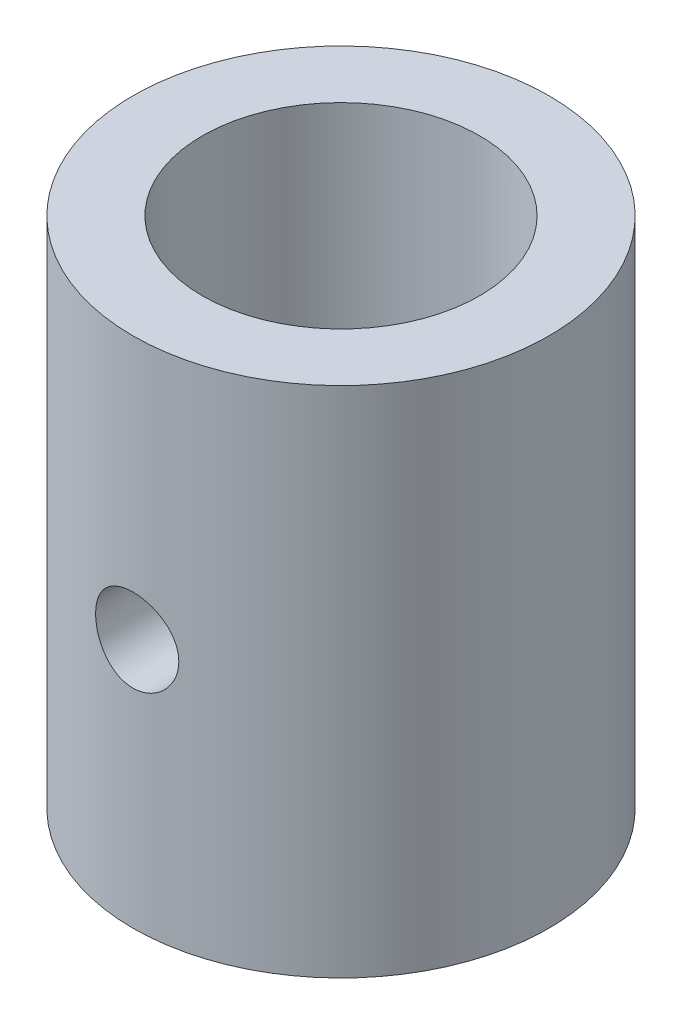
SolidWorks part; units mm, degrees
material "Plain Carbon Steel"
ref_plane "Front Plane" through (0, 0, 0) normal (0, 0, 1) x (1, 0, 0)
ref_plane "Top Plane" through (0, 0, 0) normal (0, 1, 0) x (1, 0, 0)
ref_plane "Right Plane" through (0, 0, 0) normal (1, 0, 0) x (0, 0, -1)
sketch "Bush Ring Profile Sketch" plane through (0, 0, 0) normal (0, 1, 0) x (1, 0, 0)
  circle A0 centre (0, 0) radius 15
  circle A1 centre (0, 0) radius 10
  dimension "D1" = 30
  dimension "D2" = 20
extrude "Bush Body Ø30xØ20x37" add sketch "Bush Ring Profile Sketch" along normal mid plane 37
sketch "Cross Hole Sketch" plane through (0, 0, 0) normal (0, 0, 1) x (1, 0, 0)
  line L0 (-15, -18.5) -> (15, -18.5) construction
  circle A0 centre (0, -0.5) radius 3
  dimension "D2" = 6
  dimension "D1" = 18
extrude "Cross Hole Ø6" cut sketch "Cross Hole Sketch" against normal mid plane 37
